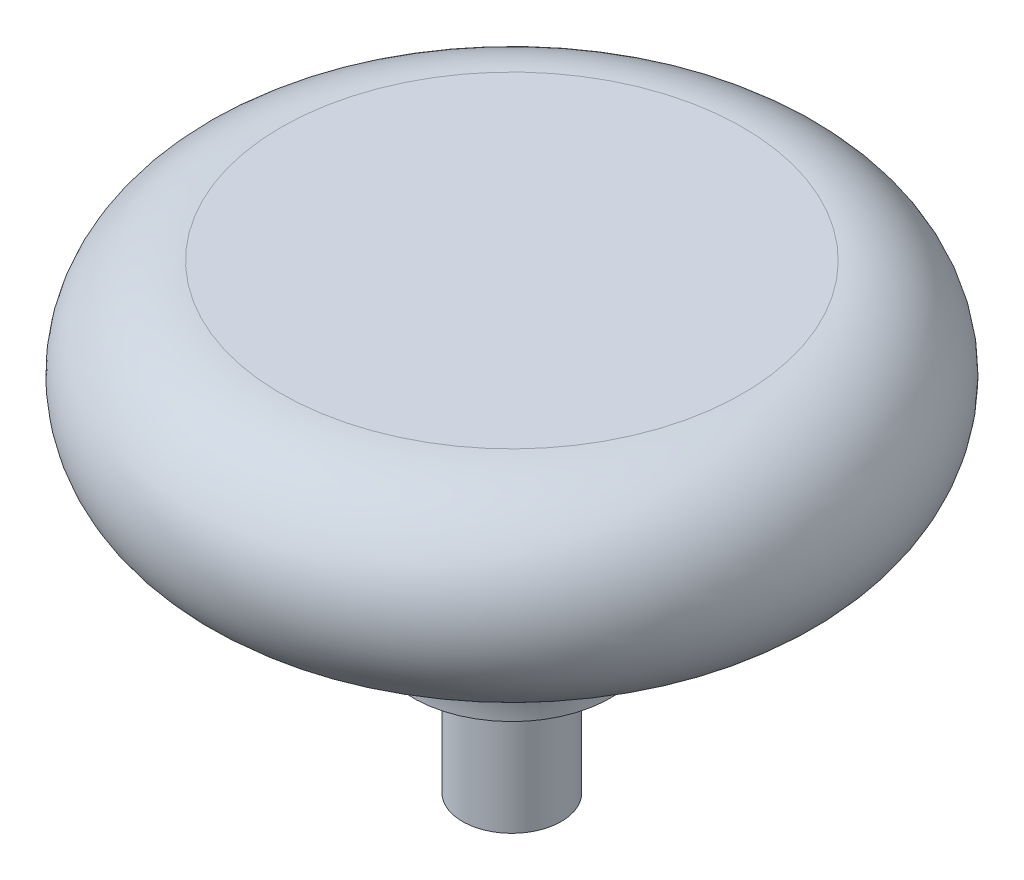
ISO-10303-21;
HEADER;
FILE_DESCRIPTION(('STEP AP214'),'2;1');
FILE_NAME('part.step','',(''),(''),'','','');
FILE_SCHEMA(('AUTOMOTIVE_DESIGN { 1 0 10303 214 1 1 1 1 }'));
ENDSEC;
DATA;
#1=APPLICATION_CONTEXT('core data for automotive mechanical design processes');
#2=APPLICATION_PROTOCOL_DEFINITION('international standard','automotive_design',2000,#1);
#3=PRODUCT_CONTEXT('',#1,'mechanical');
#4=PRODUCT('Part','Part','',(#3));
#5=PRODUCT_RELATED_PRODUCT_CATEGORY('part','',(#4));
#6=PRODUCT_DEFINITION_FORMATION('','',#4);
#7=PRODUCT_DEFINITION_CONTEXT('part definition',#1,'design');
#8=PRODUCT_DEFINITION('design','',#6,#7);
#9=PRODUCT_DEFINITION_SHAPE('','',#8);
#10=(LENGTH_UNIT() NAMED_UNIT(*) SI_UNIT(.MILLI.,.METRE.));
#11=(NAMED_UNIT(*) PLANE_ANGLE_UNIT() SI_UNIT($,.RADIAN.));
#12=(NAMED_UNIT(*) SI_UNIT($,.STERADIAN.) SOLID_ANGLE_UNIT());
#13=UNCERTAINTY_MEASURE_WITH_UNIT(LENGTH_MEASURE(1.E-05),#10,'distance_accuracy_value','');
#14=(GEOMETRIC_REPRESENTATION_CONTEXT(3) GLOBAL_UNCERTAINTY_ASSIGNED_CONTEXT((#13)) GLOBAL_UNIT_ASSIGNED_CONTEXT((#10,
#11,#12)) REPRESENTATION_CONTEXT('',''));
#15=CARTESIAN_POINT('',(0.,0.,0.));
#16=DIRECTION('',(0.,0.,1.));
#17=DIRECTION('',(1.,0.,0.));
#18=AXIS2_PLACEMENT_3D('',#15,#16,#17);
#19=CARTESIAN_POINT('',(11.1178577857786,22.22,0.));
#20=DIRECTION('',(0.,-1.,0.));
#21=DIRECTION('',(1.,0.,0.));
#22=AXIS2_PLACEMENT_3D('',#19,#20,#21);
#23=PLANE('',#22);
#24=CARTESIAN_POINT('',(0.,22.22,0.));
#25=DIRECTION('',(0.,1.,0.));
#26=DIRECTION('',(-1.,0.,0.));
#27=AXIS2_PLACEMENT_3D('',#24,#25,#26);
#28=CIRCLE('',#27,11.1178577857786);
#29=CARTESIAN_POINT('',(-11.1178577857786,22.22,0.));
#30=VERTEX_POINT('',#29);
#31=EDGE_CURVE('E10',#30,#30,#28,.T.);
#32=ORIENTED_EDGE('',*,*,#31,.T.);
#33=EDGE_LOOP('',(#32));
#34=FACE_BOUND('',#33,.T.);
#35=ADVANCED_FACE('F40',(#34),#23,.F.);
#36=CARTESIAN_POINT('',(0.,17.4600004820464,0.));
#37=DIRECTION('',(0.,1.,0.));
#38=DIRECTION('',(-1.,0.,0.));
#39=AXIS2_PLACEMENT_3D('',#36,#37,#38);
#40=TOROIDAL_SURFACE('',#39,11.12,4.76);
#41=ORIENTED_EDGE('',*,*,#31,.F.);
#42=EDGE_LOOP('',(#41));
#43=FACE_BOUND('',#42,.T.);
#44=CARTESIAN_POINT('',(0.,12.7000009640929,0.));
#45=DIRECTION('',(0.,1.,0.));
#46=DIRECTION('',(-1.,0.,0.));
#47=AXIS2_PLACEMENT_3D('',#44,#45,#46);
#48=CIRCLE('',#47,11.1178577857786);
#49=CARTESIAN_POINT('',(-11.1178577857786,12.7000009640929,0.));
#50=VERTEX_POINT('',#49);
#51=EDGE_CURVE('E43',#50,#50,#48,.T.);
#52=ORIENTED_EDGE('',*,*,#51,.T.);
#53=EDGE_LOOP('',(#52));
#54=FACE_BOUND('',#53,.T.);
#55=ADVANCED_FACE('F75',(#43,#54),#40,.T.);
#56=CARTESIAN_POINT('',(0.,6.350001607159,0.));
#57=DIRECTION('',(0.,1.,0.));
#58=DIRECTION('',(-1.,0.,0.));
#59=AXIS2_PLACEMENT_3D('',#56,#57,#58);
#60=TOROIDAL_SURFACE('',#59,11.115,6.35);
#61=ORIENTED_EDGE('',*,*,#51,.F.);
#62=EDGE_LOOP('',(#61));
#63=FACE_BOUND('',#62,.T.);
#64=CARTESIAN_POINT('',(0.,6.35000160715899,0.));
#65=DIRECTION('',(0.,1.,0.));
#66=DIRECTION('',(-1.,0.,0.));
#67=AXIS2_PLACEMENT_3D('',#64,#65,#66);
#68=CIRCLE('',#67,4.765);
#69=CARTESIAN_POINT('',(-4.765,6.35000160715899,0.));
#70=VERTEX_POINT('',#69);
#71=EDGE_CURVE('E50',#70,#70,#68,.T.);
#72=ORIENTED_EDGE('',*,*,#71,.T.);
#73=EDGE_LOOP('',(#72));
#74=FACE_BOUND('',#73,.T.);
#75=ADVANCED_FACE('F77',(#63,#74),#60,.F.);
#76=CARTESIAN_POINT('',(2.38,6.350001607159,0.));
#77=DIRECTION('',(0.,1.,0.));
#78=DIRECTION('',(-1.,0.,0.));
#79=AXIS2_PLACEMENT_3D('',#76,#77,#78);
#80=PLANE('',#79);
#81=ORIENTED_EDGE('',*,*,#71,.F.);
#82=EDGE_LOOP('',(#81));
#83=FACE_BOUND('',#82,.T.);
#84=CARTESIAN_POINT('',(0.,6.35000160715899,0.));
#85=DIRECTION('',(0.,1.,0.));
#86=DIRECTION('',(-1.,0.,0.));
#87=AXIS2_PLACEMENT_3D('',#84,#85,#86);
#88=CIRCLE('',#87,2.38);
#89=CARTESIAN_POINT('',(-2.38,6.35000160715899,0.));
#90=VERTEX_POINT('',#89);
#91=EDGE_CURVE('E51',#90,#90,#88,.T.);
#92=ORIENTED_EDGE('',*,*,#91,.T.);
#93=EDGE_LOOP('',(#92));
#94=FACE_BOUND('',#93,.T.);
#95=ADVANCED_FACE('F67',(#83,#94),#80,.F.);
#96=CARTESIAN_POINT('',(0.,22.22,0.));
#97=DIRECTION('',(0.,1.,0.));
#98=DIRECTION('',(-1.,0.,0.));
#99=AXIS2_PLACEMENT_3D('',#96,#97,#98);
#100=CYLINDRICAL_SURFACE('',#99,2.38);
#101=ORIENTED_EDGE('',*,*,#91,.F.);
#102=EDGE_LOOP('',(#101));
#103=FACE_BOUND('',#102,.T.);
#104=CARTESIAN_POINT('',(0.,0.,0.));
#105=DIRECTION('',(0.,1.,0.));
#106=DIRECTION('',(-1.,0.,0.));
#107=AXIS2_PLACEMENT_3D('',#104,#105,#106);
#108=CIRCLE('',#107,2.38);
#109=CARTESIAN_POINT('',(-2.38,0.,0.));
#110=VERTEX_POINT('',#109);
#111=EDGE_CURVE('E57',#110,#110,#108,.T.);
#112=ORIENTED_EDGE('',*,*,#111,.T.);
#113=EDGE_LOOP('',(#112));
#114=FACE_BOUND('',#113,.T.);
#115=ADVANCED_FACE('F58',(#103,#114),#100,.T.);
#116=CARTESIAN_POINT('',(0.,0.,0.));
#117=DIRECTION('',(0.,1.,0.));
#118=DIRECTION('',(-1.,0.,0.));
#119=AXIS2_PLACEMENT_3D('',#116,#117,#118);
#120=PLANE('',#119);
#121=ORIENTED_EDGE('',*,*,#111,.F.);
#122=EDGE_LOOP('',(#121));
#123=FACE_BOUND('',#122,.T.);
#124=ADVANCED_FACE('F65',(#123),#120,.F.);
#125=CLOSED_SHELL('',(#35,#55,#75,#95,#115,#124));
#126=MANIFOLD_SOLID_BREP('B2',#125);
#127=ADVANCED_BREP_SHAPE_REPRESENTATION('',(#18,#126),#14);
#128=SHAPE_DEFINITION_REPRESENTATION(#9,#127);
ENDSEC;
END-ISO-10303-21;
